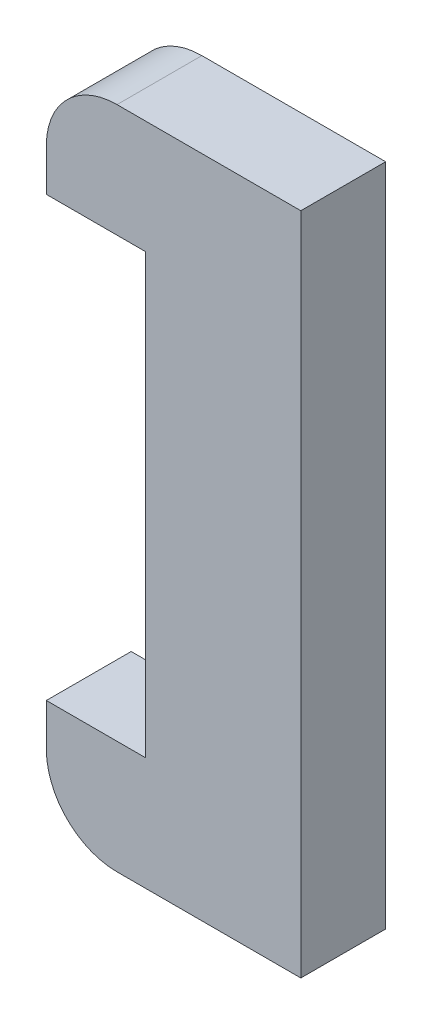
ISO-10303-21;
HEADER;
FILE_DESCRIPTION(('STEP AP214'),'2;1');
FILE_NAME('part.step','',(''),(''),'','','');
FILE_SCHEMA(('AUTOMOTIVE_DESIGN { 1 0 10303 214 1 1 1 1 }'));
ENDSEC;
DATA;
#1=APPLICATION_CONTEXT('core data for automotive mechanical design processes');
#2=APPLICATION_PROTOCOL_DEFINITION('international standard','automotive_design',2000,#1);
#3=PRODUCT_CONTEXT('',#1,'mechanical');
#4=PRODUCT('Part','Part','',(#3));
#5=PRODUCT_RELATED_PRODUCT_CATEGORY('part','',(#4));
#6=PRODUCT_DEFINITION_FORMATION('','',#4);
#7=PRODUCT_DEFINITION_CONTEXT('part definition',#1,'design');
#8=PRODUCT_DEFINITION('design','',#6,#7);
#9=PRODUCT_DEFINITION_SHAPE('','',#8);
#10=(LENGTH_UNIT() NAMED_UNIT(*) SI_UNIT(.MILLI.,.METRE.));
#11=(NAMED_UNIT(*) PLANE_ANGLE_UNIT() SI_UNIT($,.RADIAN.));
#12=(NAMED_UNIT(*) SI_UNIT($,.STERADIAN.) SOLID_ANGLE_UNIT());
#13=UNCERTAINTY_MEASURE_WITH_UNIT(LENGTH_MEASURE(1.E-05),#10,'distance_accuracy_value','');
#14=(GEOMETRIC_REPRESENTATION_CONTEXT(3) GLOBAL_UNCERTAINTY_ASSIGNED_CONTEXT((#13)) GLOBAL_UNIT_ASSIGNED_CONTEXT((#10,
#11,#12)) REPRESENTATION_CONTEXT('',''));
#15=CARTESIAN_POINT('',(0.,0.,0.));
#16=DIRECTION('',(0.,0.,1.));
#17=DIRECTION('',(1.,0.,0.));
#18=AXIS2_PLACEMENT_3D('',#15,#16,#17);
#19=CARTESIAN_POINT('',(0.,30.1777777777778,6.));
#20=DIRECTION('',(-1.,0.,0.));
#21=DIRECTION('',(0.,0.,1.));
#22=AXIS2_PLACEMENT_3D('',#19,#20,#21);
#23=PLANE('',#22);
#24=DIRECTION('',(0.,1.,0.));
#25=VECTOR('',#24,1.);
#26=CARTESIAN_POINT('',(0.,30.1777777777778,-6.));
#27=LINE('',#26,#25);
#28=CARTESIAN_POINT('',(0.,-63.8222222222222,-6.));
#29=VERTEX_POINT('',#28);
#30=CARTESIAN_POINT('',(0.,30.1777777777778,-6.));
#31=VERTEX_POINT('',#30);
#32=EDGE_CURVE('E150',#29,#31,#27,.T.);
#33=ORIENTED_EDGE('',*,*,#32,.T.);
#34=DIRECTION('',(0.,0.,-1.));
#35=VECTOR('',#34,1.);
#36=CARTESIAN_POINT('',(0.,30.1777777777778,6.));
#37=LINE('',#36,#35);
#38=CARTESIAN_POINT('',(0.,30.1777777777778,6.));
#39=VERTEX_POINT('',#38);
#40=EDGE_CURVE('E11',#39,#31,#37,.T.);
#41=ORIENTED_EDGE('',*,*,#40,.F.);
#42=DIRECTION('',(0.,1.,0.));
#43=VECTOR('',#42,1.);
#44=CARTESIAN_POINT('',(0.,30.1777777777778,6.));
#45=LINE('',#44,#43);
#46=CARTESIAN_POINT('',(0.,-63.8222222222222,6.));
#47=VERTEX_POINT('',#46);
#48=EDGE_CURVE('E164',#47,#39,#45,.T.);
#49=ORIENTED_EDGE('',*,*,#48,.F.);
#50=DIRECTION('',(0.,0.,-1.));
#51=VECTOR('',#50,1.);
#52=CARTESIAN_POINT('',(0.,-63.8222222222222,6.));
#53=LINE('',#52,#51);
#54=EDGE_CURVE('E141',#47,#29,#53,.T.);
#55=ORIENTED_EDGE('',*,*,#54,.T.);
#56=EDGE_LOOP('',(#33,#41,#49,#55));
#57=FACE_BOUND('',#56,.T.);
#58=ADVANCED_FACE('F39',(#57),#23,.F.);
#59=CARTESIAN_POINT('',(-26.,30.1777777777778,6.));
#60=DIRECTION('',(0.,-1.,0.));
#61=DIRECTION('',(1.,0.,0.));
#62=AXIS2_PLACEMENT_3D('',#59,#60,#61);
#63=PLANE('',#62);
#64=DIRECTION('',(-1.,0.,0.));
#65=VECTOR('',#64,1.);
#66=CARTESIAN_POINT('',(-26.,30.1777777777778,-6.));
#67=LINE('',#66,#65);
#68=CARTESIAN_POINT('',(-26.,30.1777777777778,-6.));
#69=VERTEX_POINT('',#68);
#70=EDGE_CURVE('E147',#31,#69,#67,.T.);
#71=ORIENTED_EDGE('',*,*,#70,.T.);
#72=DIRECTION('',(0.,0.,-1.));
#73=VECTOR('',#72,1.);
#74=CARTESIAN_POINT('',(-26.,30.1777777777778,6.));
#75=LINE('',#74,#73);
#76=CARTESIAN_POINT('',(-26.,30.1777777777778,6.));
#77=VERTEX_POINT('',#76);
#78=EDGE_CURVE('E50',#77,#69,#75,.T.);
#79=ORIENTED_EDGE('',*,*,#78,.F.);
#80=DIRECTION('',(-1.,0.,0.));
#81=VECTOR('',#80,1.);
#82=CARTESIAN_POINT('',(-26.,30.1777777777778,6.));
#83=LINE('',#82,#81);
#84=EDGE_CURVE('E102',#39,#77,#83,.T.);
#85=ORIENTED_EDGE('',*,*,#84,.F.);
#86=ORIENTED_EDGE('',*,*,#40,.T.);
#87=EDGE_LOOP('',(#71,#79,#85,#86));
#88=FACE_BOUND('',#87,.T.);
#89=ADVANCED_FACE('F212',(#88),#63,.F.);
#90=CARTESIAN_POINT('',(-26.,20.1777777777778,6.));
#91=DIRECTION('',(0.,0.,-1.));
#92=DIRECTION('',(-1.,0.,0.));
#93=AXIS2_PLACEMENT_3D('',#90,#91,#92);
#94=CYLINDRICAL_SURFACE('',#93,10.);
#95=CARTESIAN_POINT('',(-26.,20.1777777777778,-6.));
#96=DIRECTION('',(0.,0.,1.));
#97=DIRECTION('',(1.,0.,0.));
#98=AXIS2_PLACEMENT_3D('',#95,#96,#97);
#99=CIRCLE('',#98,10.);
#100=CARTESIAN_POINT('',(-36.,20.1777777777778,-6.));
#101=VERTEX_POINT('',#100);
#102=EDGE_CURVE('E155',#69,#101,#99,.T.);
#103=ORIENTED_EDGE('',*,*,#102,.T.);
#104=DIRECTION('',(0.,0.,-1.));
#105=VECTOR('',#104,1.);
#106=CARTESIAN_POINT('',(-36.,20.1777777777778,6.));
#107=LINE('',#106,#105);
#108=CARTESIAN_POINT('',(-36.,20.1777777777778,6.));
#109=VERTEX_POINT('',#108);
#110=EDGE_CURVE('E179',#109,#101,#107,.T.);
#111=ORIENTED_EDGE('',*,*,#110,.F.);
#112=CARTESIAN_POINT('',(-26.,20.1777777777778,6.));
#113=DIRECTION('',(0.,0.,1.));
#114=DIRECTION('',(1.,0.,0.));
#115=AXIS2_PLACEMENT_3D('',#112,#113,#114);
#116=CIRCLE('',#115,10.);
#117=EDGE_CURVE('E187',#77,#109,#116,.T.);
#118=ORIENTED_EDGE('',*,*,#117,.F.);
#119=ORIENTED_EDGE('',*,*,#78,.T.);
#120=EDGE_LOOP('',(#103,#111,#118,#119));
#121=FACE_BOUND('',#120,.T.);
#122=ADVANCED_FACE('F184',(#121),#94,.T.);
#123=CARTESIAN_POINT('',(-36.,14.1777777777778,6.));
#124=DIRECTION('',(1.,0.,0.));
#125=DIRECTION('',(0.,0.,-1.));
#126=AXIS2_PLACEMENT_3D('',#123,#124,#125);
#127=PLANE('',#126);
#128=DIRECTION('',(0.,-1.,0.));
#129=VECTOR('',#128,1.);
#130=CARTESIAN_POINT('',(-36.,14.1777777777778,-6.));
#131=LINE('',#130,#129);
#132=CARTESIAN_POINT('',(-36.,14.1777777777778,-6.));
#133=VERTEX_POINT('',#132);
#134=EDGE_CURVE('E152',#101,#133,#131,.T.);
#135=ORIENTED_EDGE('',*,*,#134,.T.);
#136=DIRECTION('',(0.,0.,-1.));
#137=VECTOR('',#136,1.);
#138=CARTESIAN_POINT('',(-36.,14.1777777777778,6.));
#139=LINE('',#138,#137);
#140=CARTESIAN_POINT('',(-36.,14.1777777777778,6.));
#141=VERTEX_POINT('',#140);
#142=EDGE_CURVE('E173',#141,#133,#139,.T.);
#143=ORIENTED_EDGE('',*,*,#142,.F.);
#144=DIRECTION('',(0.,-1.,0.));
#145=VECTOR('',#144,1.);
#146=CARTESIAN_POINT('',(-36.,14.1777777777778,6.));
#147=LINE('',#146,#145);
#148=EDGE_CURVE('E204',#109,#141,#147,.T.);
#149=ORIENTED_EDGE('',*,*,#148,.F.);
#150=ORIENTED_EDGE('',*,*,#110,.T.);
#151=EDGE_LOOP('',(#135,#143,#149,#150));
#152=FACE_BOUND('',#151,.T.);
#153=ADVANCED_FACE('F193',(#152),#127,.F.);
#154=CARTESIAN_POINT('',(-22.,14.1777777777778,6.));
#155=DIRECTION('',(0.,1.,0.));
#156=DIRECTION('',(-1.,0.,0.));
#157=AXIS2_PLACEMENT_3D('',#154,#155,#156);
#158=PLANE('',#157);
#159=DIRECTION('',(1.,0.,0.));
#160=VECTOR('',#159,1.);
#161=CARTESIAN_POINT('',(-22.,14.1777777777778,-6.));
#162=LINE('',#161,#160);
#163=CARTESIAN_POINT('',(-22.,14.1777777777778,-6.));
#164=VERTEX_POINT('',#163);
#165=EDGE_CURVE('E156',#133,#164,#162,.T.);
#166=ORIENTED_EDGE('',*,*,#165,.T.);
#167=DIRECTION('',(0.,0.,-1.));
#168=VECTOR('',#167,1.);
#169=CARTESIAN_POINT('',(-22.,14.1777777777778,6.));
#170=LINE('',#169,#168);
#171=CARTESIAN_POINT('',(-22.,14.1777777777778,6.));
#172=VERTEX_POINT('',#171);
#173=EDGE_CURVE('E175',#172,#164,#170,.T.);
#174=ORIENTED_EDGE('',*,*,#173,.F.);
#175=DIRECTION('',(1.,0.,0.));
#176=VECTOR('',#175,1.);
#177=CARTESIAN_POINT('',(-22.,14.1777777777778,6.));
#178=LINE('',#177,#176);
#179=EDGE_CURVE('E203',#141,#172,#178,.T.);
#180=ORIENTED_EDGE('',*,*,#179,.F.);
#181=ORIENTED_EDGE('',*,*,#142,.T.);
#182=EDGE_LOOP('',(#166,#174,#180,#181));
#183=FACE_BOUND('',#182,.T.);
#184=ADVANCED_FACE('F200',(#183),#158,.F.);
#185=CARTESIAN_POINT('',(-22.,-47.8222222222222,6.));
#186=DIRECTION('',(1.,0.,0.));
#187=DIRECTION('',(0.,1.,0.));
#188=AXIS2_PLACEMENT_3D('',#185,#186,#187);
#189=PLANE('',#188);
#190=DIRECTION('',(0.,-1.,0.));
#191=VECTOR('',#190,1.);
#192=CARTESIAN_POINT('',(-22.,-47.8222222222222,-6.));
#193=LINE('',#192,#191);
#194=CARTESIAN_POINT('',(-22.,-47.8222222222222,-6.));
#195=VERTEX_POINT('',#194);
#196=EDGE_CURVE('E158',#164,#195,#193,.T.);
#197=ORIENTED_EDGE('',*,*,#196,.T.);
#198=DIRECTION('',(0.,0.,-1.));
#199=VECTOR('',#198,1.);
#200=CARTESIAN_POINT('',(-22.,-47.8222222222222,6.));
#201=LINE('',#200,#199);
#202=CARTESIAN_POINT('',(-22.,-47.8222222222222,6.));
#203=VERTEX_POINT('',#202);
#204=EDGE_CURVE('E166',#203,#195,#201,.T.);
#205=ORIENTED_EDGE('',*,*,#204,.F.);
#206=DIRECTION('',(0.,-1.,0.));
#207=VECTOR('',#206,1.);
#208=CARTESIAN_POINT('',(-22.,-47.8222222222222,6.));
#209=LINE('',#208,#207);
#210=EDGE_CURVE('E201',#172,#203,#209,.T.);
#211=ORIENTED_EDGE('',*,*,#210,.F.);
#212=ORIENTED_EDGE('',*,*,#173,.T.);
#213=EDGE_LOOP('',(#197,#205,#211,#212));
#214=FACE_BOUND('',#213,.T.);
#215=ADVANCED_FACE('F227',(#214),#189,.F.);
#216=CARTESIAN_POINT('',(-36.,-47.8222222222222,6.));
#217=DIRECTION('',(0.,-1.,0.));
#218=DIRECTION('',(0.,0.,-1.));
#219=AXIS2_PLACEMENT_3D('',#216,#217,#218);
#220=PLANE('',#219);
#221=DIRECTION('',(-1.,0.,0.));
#222=VECTOR('',#221,1.);
#223=CARTESIAN_POINT('',(-36.,-47.8222222222222,-6.));
#224=LINE('',#223,#222);
#225=CARTESIAN_POINT('',(-36.,-47.8222222222222,-6.));
#226=VERTEX_POINT('',#225);
#227=EDGE_CURVE('E159',#195,#226,#224,.T.);
#228=ORIENTED_EDGE('',*,*,#227,.T.);
#229=DIRECTION('',(0.,0.,-1.));
#230=VECTOR('',#229,1.);
#231=CARTESIAN_POINT('',(-36.,-47.8222222222222,6.));
#232=LINE('',#231,#230);
#233=CARTESIAN_POINT('',(-36.,-47.8222222222222,6.));
#234=VERTEX_POINT('',#233);
#235=EDGE_CURVE('E139',#234,#226,#232,.T.);
#236=ORIENTED_EDGE('',*,*,#235,.F.);
#237=DIRECTION('',(-1.,0.,0.));
#238=VECTOR('',#237,1.);
#239=CARTESIAN_POINT('',(-36.,-47.8222222222222,6.));
#240=LINE('',#239,#238);
#241=EDGE_CURVE('E129',#203,#234,#240,.T.);
#242=ORIENTED_EDGE('',*,*,#241,.F.);
#243=ORIENTED_EDGE('',*,*,#204,.T.);
#244=EDGE_LOOP('',(#228,#236,#242,#243));
#245=FACE_BOUND('',#244,.T.);
#246=ADVANCED_FACE('F226',(#245),#220,.F.);
#247=CARTESIAN_POINT('',(-36.,-53.8222222222222,6.));
#248=DIRECTION('',(1.,0.,0.));
#249=DIRECTION('',(0.,0.,-1.));
#250=AXIS2_PLACEMENT_3D('',#247,#248,#249);
#251=PLANE('',#250);
#252=DIRECTION('',(0.,-1.,0.));
#253=VECTOR('',#252,1.);
#254=CARTESIAN_POINT('',(-36.,-53.8222222222222,-6.));
#255=LINE('',#254,#253);
#256=CARTESIAN_POINT('',(-36.,-53.8222222222222,-6.));
#257=VERTEX_POINT('',#256);
#258=EDGE_CURVE('E140',#226,#257,#255,.T.);
#259=ORIENTED_EDGE('',*,*,#258,.T.);
#260=DIRECTION('',(0.,0.,-1.));
#261=VECTOR('',#260,1.);
#262=CARTESIAN_POINT('',(-36.,-53.8222222222222,6.));
#263=LINE('',#262,#261);
#264=CARTESIAN_POINT('',(-36.,-53.8222222222222,6.));
#265=VERTEX_POINT('',#264);
#266=EDGE_CURVE('E131',#265,#257,#263,.T.);
#267=ORIENTED_EDGE('',*,*,#266,.F.);
#268=DIRECTION('',(0.,-1.,0.));
#269=VECTOR('',#268,1.);
#270=CARTESIAN_POINT('',(-36.,-53.8222222222222,6.));
#271=LINE('',#270,#269);
#272=EDGE_CURVE('E124',#234,#265,#271,.T.);
#273=ORIENTED_EDGE('',*,*,#272,.F.);
#274=ORIENTED_EDGE('',*,*,#235,.T.);
#275=EDGE_LOOP('',(#259,#267,#273,#274));
#276=FACE_BOUND('',#275,.T.);
#277=ADVANCED_FACE('F133',(#276),#251,.F.);
#278=CARTESIAN_POINT('',(-26.,-53.8222222222222,6.));
#279=DIRECTION('',(0.,0.,-1.));
#280=DIRECTION('',(-1.,0.,0.));
#281=AXIS2_PLACEMENT_3D('',#278,#279,#280);
#282=CYLINDRICAL_SURFACE('',#281,10.);
#283=CARTESIAN_POINT('',(-26.,-53.8222222222222,-6.));
#284=DIRECTION('',(0.,0.,1.));
#285=DIRECTION('',(-1.,0.,0.));
#286=AXIS2_PLACEMENT_3D('',#283,#284,#285);
#287=CIRCLE('',#286,10.);
#288=CARTESIAN_POINT('',(-25.9999999999999,-63.8222222222222,-6.));
#289=VERTEX_POINT('',#288);
#290=EDGE_CURVE('E89',#257,#289,#287,.T.);
#291=ORIENTED_EDGE('',*,*,#290,.T.);
#292=DIRECTION('',(0.,0.,-1.));
#293=VECTOR('',#292,1.);
#294=CARTESIAN_POINT('',(-25.9999999999999,-63.8222222222222,6.));
#295=LINE('',#294,#293);
#296=CARTESIAN_POINT('',(-25.9999999999999,-63.8222222222222,6.));
#297=VERTEX_POINT('',#296);
#298=EDGE_CURVE('E136',#297,#289,#295,.T.);
#299=ORIENTED_EDGE('',*,*,#298,.F.);
#300=CARTESIAN_POINT('',(-26.,-53.8222222222222,6.));
#301=DIRECTION('',(0.,0.,1.));
#302=DIRECTION('',(-1.,0.,0.));
#303=AXIS2_PLACEMENT_3D('',#300,#301,#302);
#304=CIRCLE('',#303,10.);
#305=EDGE_CURVE('E130',#265,#297,#304,.T.);
#306=ORIENTED_EDGE('',*,*,#305,.F.);
#307=ORIENTED_EDGE('',*,*,#266,.T.);
#308=EDGE_LOOP('',(#291,#299,#306,#307));
#309=FACE_BOUND('',#308,.T.);
#310=ADVANCED_FACE('F143',(#309),#282,.T.);
#311=CARTESIAN_POINT('',(0.,-63.8222222222222,6.));
#312=DIRECTION('',(0.,1.,0.));
#313=DIRECTION('',(0.,0.,1.));
#314=AXIS2_PLACEMENT_3D('',#311,#312,#313);
#315=PLANE('',#314);
#316=DIRECTION('',(1.,0.,0.));
#317=VECTOR('',#316,1.);
#318=CARTESIAN_POINT('',(0.,-63.8222222222222,-6.));
#319=LINE('',#318,#317);
#320=EDGE_CURVE('E96',#289,#29,#319,.T.);
#321=ORIENTED_EDGE('',*,*,#320,.T.);
#322=ORIENTED_EDGE('',*,*,#54,.F.);
#323=DIRECTION('',(1.,0.,0.));
#324=VECTOR('',#323,1.);
#325=CARTESIAN_POINT('',(0.,-63.8222222222222,6.));
#326=LINE('',#325,#324);
#327=EDGE_CURVE('E54',#297,#47,#326,.T.);
#328=ORIENTED_EDGE('',*,*,#327,.F.);
#329=ORIENTED_EDGE('',*,*,#298,.T.);
#330=EDGE_LOOP('',(#321,#322,#328,#329));
#331=FACE_BOUND('',#330,.T.);
#332=ADVANCED_FACE('F236',(#331),#315,.F.);
#333=CARTESIAN_POINT('',(-26.,-53.8222222222222,6.));
#334=DIRECTION('',(0.,0.,-1.));
#335=DIRECTION('',(-1.,0.,0.));
#336=AXIS2_PLACEMENT_3D('',#333,#334,#335);
#337=PLANE('',#336);
#338=ORIENTED_EDGE('',*,*,#48,.T.);
#339=ORIENTED_EDGE('',*,*,#84,.T.);
#340=ORIENTED_EDGE('',*,*,#117,.T.);
#341=ORIENTED_EDGE('',*,*,#148,.T.);
#342=ORIENTED_EDGE('',*,*,#179,.T.);
#343=ORIENTED_EDGE('',*,*,#210,.T.);
#344=ORIENTED_EDGE('',*,*,#241,.T.);
#345=ORIENTED_EDGE('',*,*,#272,.T.);
#346=ORIENTED_EDGE('',*,*,#305,.T.);
#347=ORIENTED_EDGE('',*,*,#327,.T.);
#348=EDGE_LOOP('',(#338,#339,#340,#341,#342,#343,#344,#345,#346,#347));
#349=FACE_BOUND('',#348,.T.);
#350=ADVANCED_FACE('F123',(#349),#337,.F.);
#351=CARTESIAN_POINT('',(-26.,-53.8222222222222,-6.));
#352=DIRECTION('',(0.,0.,-1.));
#353=DIRECTION('',(-1.,0.,0.));
#354=AXIS2_PLACEMENT_3D('',#351,#352,#353);
#355=PLANE('',#354);
#356=ORIENTED_EDGE('',*,*,#32,.F.);
#357=ORIENTED_EDGE('',*,*,#320,.F.);
#358=ORIENTED_EDGE('',*,*,#290,.F.);
#359=ORIENTED_EDGE('',*,*,#258,.F.);
#360=ORIENTED_EDGE('',*,*,#227,.F.);
#361=ORIENTED_EDGE('',*,*,#196,.F.);
#362=ORIENTED_EDGE('',*,*,#165,.F.);
#363=ORIENTED_EDGE('',*,*,#134,.F.);
#364=ORIENTED_EDGE('',*,*,#102,.F.);
#365=ORIENTED_EDGE('',*,*,#70,.F.);
#366=EDGE_LOOP('',(#356,#357,#358,#359,#360,#361,#362,#363,#364,#365));
#367=FACE_BOUND('',#366,.T.);
#368=ADVANCED_FACE('F188',(#367),#355,.T.);
#369=CLOSED_SHELL('',(#58,#89,#122,#153,#184,#215,#246,#277,#310,#332,#350,#368));
#370=MANIFOLD_SOLID_BREP('B2',#369);
#371=ADVANCED_BREP_SHAPE_REPRESENTATION('',(#18,#370),#14);
#372=SHAPE_DEFINITION_REPRESENTATION(#9,#371);
ENDSEC;
END-ISO-10303-21;
